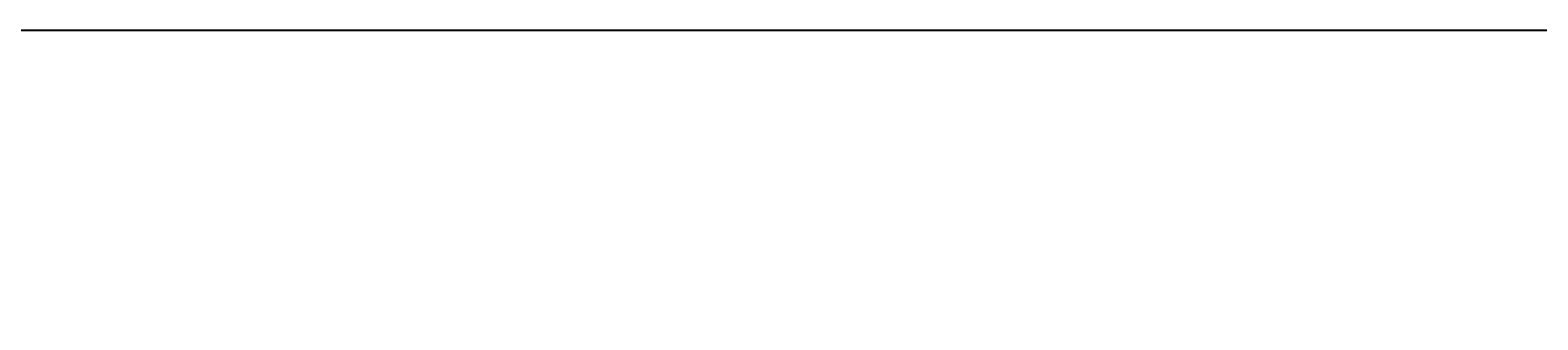
# Model space of a CAD drawing. Units: inches. Extents: x 1885 to 2748, y 783 to 2421.
# Tile 13 of 117: x 2065 to 2102, y 1050 to 1058. Entities that reach past the tile are written whole.
import ezdxf

# ---------------------------------------------------------------- set-up
doc = ezdxf.new("R2010")
doc.units = ezdxf.units.IN
doc.layers.add('A-ANNO-DIMS', color=2, linetype='Continuous', lineweight=18)
doc.layers.add('A-FLOR-BALC', color=7, linetype='Continuous', lineweight=25)
doc.styles.get("Standard").update_dxf_attribs({"font": 'arial.ttf'})
doc.dimstyles.get("Standard").update_dxf_attribs({"dimtxt": 0.18, "dimasz": 0.18, "dimexe": 0.18, "dimexo": 0.0625, "dimgap": 0.09, "dimtad": 0, "dimtih": 1, "dimtoh": 1, "dimdec": 4, "dimzin": 0, "dimdsep": 46, "dimtxsty": 'Standard', "dimcen": 0.09, "dimadec": 0, "dimazin": 0, "dimtfac": 1, "dimtdec": 4, "dimtofl": 0, "dimtmove": 0, "dimatfit": 3, "dimfxl": 1, "dimtolj": 1, "dimtzin": 0, "dimarcsym": 0})

# ---------------------------------------------------------------- blocks, each defined once
blk = doc.blocks.new('*D43')
at = {"layer": 'A-ANNO-DIMS', "color": 0, "lineweight": -2, "transparency": 16777216}
for p, q in [((1971.274, 1057.443), (1971.274, 922.479)), ((2618.274, 1057.443), (2618.274, 922.479)), ((1971.454, 922.659), (2294.484, 922.659)), ((2618.094, 922.659), (2295.063, 922.659))]:
    blk.add_line(p, q, dxfattribs=at)
at = {"layer": 'A-ANNO-DIMS', "color": 0, "transparency": 16777216}
for points in [[(1971.454, 922.689), (1971.454, 922.629), (1971.274, 922.659)], [(2618.094, 922.689), (2618.094, 922.629), (2618.274, 922.659)]]:
    blk.add_solid(points, dxfattribs=at)
at = {"layer": 'Defpoints', "color": 0, "transparency": 16777216}
for p in [(1971.274, 1057.506), (2618.274, 1057.506), (2618.274, 922.659)]:
    blk.add_point(p, dxfattribs=at)
at = {"layer": 'A-ANNO-DIMS', "color": 0, "transparency": 16777216, "insert": (2294.774, 922.659), "char_height": 0.18, "attachment_point": 5}
blk.add_mtext('\\A1;647', dxfattribs=at)

msp = doc.modelspace()

# ---------------------------------------------------------------- linework, layer by layer
at = {"layer": 'A-FLOR-BALC'}
msp.add_line((1971.274, 1057.506), (2112.274, 1057.506), dxfattribs=at)

# ---------------------------------------------------------------- dimensions: what is measured, and where the dimension line sits
at = {"layer": 'A-ANNO-DIMS'}
dim = msp.add_linear_dim(base=(2618.274, 922.659), p1=(1971.274, 1057.506), p2=(2618.274, 1057.506), dimstyle='Standard', override={"dimdec": 0, "dimlfac": 1, "dimrnd": 0, "dimzin": 0, "dimdsep": 46, "dimlunit": 2}, dxfattribs=at)
dim.commit()
dim.dimension.update_dxf_attribs({"geometry": '*D43', "text_midpoint": (2294.774, 922.659)})

doc.saveas('drawing.dxf')
